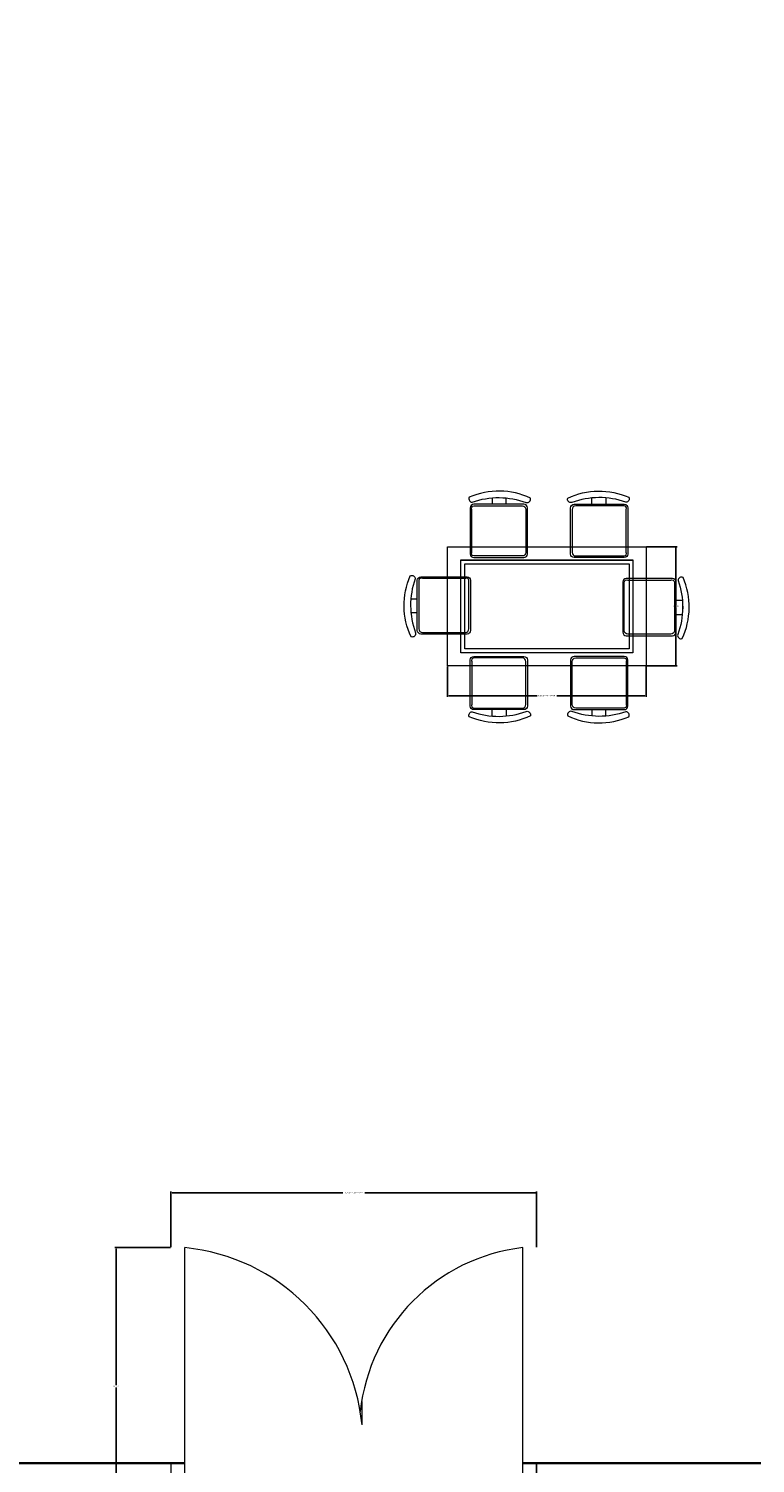
# Model space of a CAD drawing. Units: inches. Extents: x 1824 to 3509, y 619 to 2294.
# Tile 5 of 12: x 2202 to 2308, y 1115 to 1325. Entities that reach past the tile are written whole.
import ezdxf

# ---------------------------------------------------------------- set-up
doc = ezdxf.new("R2010")
doc.units = ezdxf.units.IN
for name, color, linetype, lineweight in [('A-ANNO-DIMS', 2, 'Continuous', 18), ('A-DOOR', 3, 'Continuous', 18), ('A-FURN', 8, 'Continuous', 13), ('A-WALL', 7, 'Continuous', 35)]:
    doc.layers.add(name, color=color, linetype=linetype, lineweight=lineweight)
doc.styles.get("Standard").update_dxf_attribs({"font": 'arial.ttf'})
doc.dimstyles.get("Standard").update_dxf_attribs({"dimtxt": 0.18, "dimasz": 0.18, "dimexe": 0.18, "dimexo": 0.0625, "dimgap": 0.09, "dimtad": 0, "dimtih": 1, "dimtoh": 1, "dimdec": 4, "dimzin": 0, "dimdsep": 46, "dimtxsty": 'Standard', "dimcen": 0.09, "dimadec": 0, "dimazin": 0, "dimtfac": 1, "dimtdec": 4, "dimtofl": 0, "dimtmove": 0, "dimatfit": 3, "dimfxl": 1, "dimtolj": 1, "dimtzin": 0, "dimarcsym": 0})

# ---------------------------------------------------------------- blocks, each defined once
blk = doc.blocks.new('DOOR-LOUNGE-PAIR')
for p, q in [((2, 4.5), (2, 40.5)), ((51.41, 4.5), (51.41, 40.5)), ((27.9, 14.63), (27.9, 18.05)), ((0, 9), (0, 0)), ((53.41, 0), (53.41, 9)), ((53.41, 9), (53.41, 4.5)), ((0, 0), (0, 4.5)), ((0, 4.5), (2, 4.5)), ((53.41, 4.5), (51.41, 4.5)), ((53.41, 4.5), (53.41, 4.5))]:
    blk.add_line(p, q)
for centre, radius, start, end in [((-0.78, 11.81), 28.82, 5.6014, 84.4566), ((54.5, 13.67), 27.01, 96.5732, 173.8895)]:
    blk.add_arc(centre, radius, start, end)
blk = doc.blocks.new('DINING-TABLE-PLAN')
for points in [[(0, 17.41), (29.01, 17.41), (29.01, 0), (0, 0)], [(1.93, 15.47), (27.08, 15.47), (27.08, 1.93), (1.93, 1.93)], [(2.51, 14.89), (26.5, 14.89), (26.5, 2.51), (2.51, 2.51)]]:
    blk.add_lwpolyline(points, close=True)
blk = doc.blocks.new('*D74')
at = {"layer": 'A-ANNO-DIMS', "color": 0, "lineweight": -2, "transparency": 16777216}
for p, q in [((2222.44, 1146.66), (2222.44, 1154.79)), ((2222.62, 1154.61), (2247.56, 1154.61)), ((2275.67, 1154.61), (2250.73, 1154.61)), ((2275.85, 1146.66), (2275.85, 1154.79))]:
    blk.add_line(p, q, dxfattribs=at)
at = {"layer": 'A-ANNO-DIMS', "color": 0, "transparency": 16777216}
for points in [[(2222.62, 1154.64), (2222.62, 1154.58), (2222.44, 1154.61)], [(2275.67, 1154.64), (2275.67, 1154.58), (2275.85, 1154.61)]]:
    blk.add_solid(points, dxfattribs=at)
at = {"layer": 'Defpoints', "color": 0, "transparency": 16777216}
for p in [(2275.85, 1154.61), (2222.44, 1146.6), (2275.85, 1146.6)]:
    blk.add_point(p, dxfattribs=at)
at = {"layer": 'A-ANNO-DIMS', "color": 0, "transparency": 16777216, "insert": (2249.14, 1154.61), "char_height": 0.18, "attachment_point": 5}
blk.add_mtext('\\A1;LOUNGE DOORS 53 TYP.', dxfattribs=at)
blk = doc.blocks.new('*D75')
at = {"layer": 'A-ANNO-DIMS', "color": 0, "lineweight": -2, "transparency": 16777216}
for p, q in [((2222.38, 1146.6), (2214.25, 1146.6)), ((2214.43, 1146.42), (2214.43, 1126.53)), ((2214.43, 1106.28), (2214.43, 1126.17)), ((2222.38, 1106.1), (2214.25, 1106.1))]:
    blk.add_line(p, q, dxfattribs=at)
at = {"layer": 'A-ANNO-DIMS', "color": 0, "transparency": 16777216}
for points in [[(2214.4, 1146.42), (2214.46, 1146.42), (2214.43, 1146.6)], [(2214.4, 1106.28), (2214.46, 1106.28), (2214.43, 1106.1)]]:
    blk.add_solid(points, dxfattribs=at)
at = {"layer": 'Defpoints', "color": 0, "transparency": 16777216}
for p in [(2214.43, 1146.6), (2222.44, 1146.6), (2222.44, 1106.1)]:
    blk.add_point(p, dxfattribs=at)
at = {"layer": 'A-ANNO-DIMS', "color": 0, "transparency": 16777216, "insert": (2214.43, 1126.35), "char_height": 0.18, "attachment_point": 5}
blk.add_mtext('\\A1;41 TYP.', dxfattribs=at)
blk = doc.blocks.new('*D90')
at = {"layer": 'A-ANNO-DIMS', "color": 0, "lineweight": -2, "transparency": 16777216}
for p, q in [((2262.84, 1231.49), (2262.84, 1227.02)), ((2291.85, 1231.49), (2291.85, 1227.02)), ((2263.02, 1227.2), (2275.91, 1227.2)), ((2291.67, 1227.2), (2278.78, 1227.2))]:
    blk.add_line(p, q, dxfattribs=at)
at = {"layer": 'A-ANNO-DIMS', "color": 0, "transparency": 16777216}
for points in [[(2263.02, 1227.23), (2263.02, 1227.17), (2262.84, 1227.2)], [(2291.67, 1227.23), (2291.67, 1227.17), (2291.85, 1227.2)]]:
    blk.add_solid(points, dxfattribs=at)
at = {"layer": 'Defpoints', "color": 0, "transparency": 16777216}
for p in [(2262.84, 1231.55), (2291.85, 1231.55), (2291.85, 1227.2)]:
    blk.add_point(p, dxfattribs=at)
at = {"layer": 'A-ANNO-DIMS', "color": 0, "transparency": 16777216, "insert": (2277.35, 1227.2), "char_height": 0.18, "attachment_point": 5}
blk.add_mtext('\\A1;DINING TABLE 29 TYP.', dxfattribs=at)
blk = doc.blocks.new('*D91')
at = {"layer": 'A-ANNO-DIMS', "color": 0, "lineweight": -2, "transparency": 16777216}
for p, q in [((2291.91, 1248.96), (2296.38, 1248.96)), ((2296.2, 1248.78), (2296.2, 1240.44)), ((2296.2, 1231.73), (2296.2, 1240.08)), ((2291.91, 1231.55), (2296.38, 1231.55))]:
    blk.add_line(p, q, dxfattribs=at)
at = {"layer": 'A-ANNO-DIMS', "color": 0, "transparency": 16777216}
for points in [[(2296.17, 1248.78), (2296.23, 1248.78), (2296.2, 1248.96)], [(2296.17, 1231.73), (2296.23, 1231.73), (2296.2, 1231.55)]]:
    blk.add_solid(points, dxfattribs=at)
at = {"layer": 'Defpoints', "color": 0, "transparency": 16777216}
for p in [(2291.85, 1248.96), (2296.2, 1248.96), (2291.85, 1231.55)]:
    blk.add_point(p, dxfattribs=at)
at = {"layer": 'A-ANNO-DIMS', "color": 0, "transparency": 16777216, "insert": (2296.2, 1240.26), "char_height": 0.18, "attachment_point": 5}
blk.add_mtext('\\A1;17 TYP.', dxfattribs=at)
blk = doc.blocks.new('*D94')
at = {"layer": 'A-ANNO-DIMS', "color": 0, "lineweight": -2, "transparency": 16777216}
for p, q in [((1949.09, 1049.16), (1949.09, 1668.03)), ((1949.27, 1667.85), (2235.8, 1667.85)), ((2522.91, 1667.85), (2236.38, 1667.85)), ((2523.09, 1622.16), (2523.09, 1668.03))]:
    blk.add_line(p, q, dxfattribs=at)
at = {"layer": 'A-ANNO-DIMS', "color": 0, "transparency": 16777216}
for points in [[(1949.27, 1667.88), (1949.27, 1667.82), (1949.09, 1667.85)], [(2522.91, 1667.88), (2522.91, 1667.82), (2523.09, 1667.85)]]:
    blk.add_solid(points, dxfattribs=at)
at = {"layer": 'Defpoints', "color": 0, "transparency": 16777216}
for p in [(2523.09, 1667.85), (2523.09, 1622.1), (1949.09, 1049.1)]:
    blk.add_point(p, dxfattribs=at)
at = {"layer": 'A-ANNO-DIMS', "color": 0, "transparency": 16777216, "insert": (2236.09, 1667.85), "char_height": 0.18, "attachment_point": 5}
blk.add_mtext('\\A1;574', dxfattribs=at)

msp = doc.modelspace()

# ---------------------------------------------------------------- linework, layer by layer
at = {"layer": 'A-FURN'}
for points in [[(2266.4285, 1255.4711, -0.17580919), (2274.3302, 1255.4113, 0.57839206), (2274.9288, 1256.0695, 0.21452438), (2266.0094, 1256.1892, 0.55201397), (2266.4285, 1255.4711, -0.06507904)], [(2266.4285, 1255.4708, -0.17580919), (2274.3302, 1255.411, 0.57839206), (2274.9288, 1256.0692, 0.21452438), (2266.0094, 1256.1889, 0.55201397), (2266.4285, 1255.4708, -0.06507904)], [(2280.9824, 1255.4113, -0.57839206), (2280.3838, 1256.0695, -0.21452438), (2289.3031, 1256.1892, -0.55201397), (2288.8841, 1255.4711, 0.1758092), (2280.9824, 1255.4113)], [(2280.9824, 1255.411, -0.57839206), (2280.3838, 1256.0692, -0.21452438), (2289.3031, 1256.1889, -0.55201397), (2288.8841, 1255.4708, 0.1758092), (2280.9824, 1255.411)], [(2273.9949, 1255.154), (2266.6593, 1255.154, 0.41421356), (2266.146, 1254.6408), (2266.146, 1247.8958, 0.41421356), (2266.6593, 1247.3825), (2273.9949, 1247.3825, 0.41421356), (2274.5081, 1247.8958), (2274.5081, 1254.6408, 0.41421356), (2273.9949, 1255.154)], [(2273.9949, 1255.1537), (2266.6593, 1255.1537, 0.41421356), (2266.1461, 1254.6405), (2266.1461, 1247.8954, 0.41421356), (2266.6593, 1247.3822), (2273.9949, 1247.3822, 0.41421356), (2274.5082, 1247.8954), (2274.5082, 1254.6405, 0.41421356), (2273.9949, 1255.1537)], [(2271.4183, 1255.154), (2271.4183, 1256.0817, -0.06475861)], [(2271.4183, 1255.1537), (2271.4183, 1256.0814, -0.06475861)], [(2288.6533, 1255.154, -0.41421356), (2289.1665, 1254.6408), (2289.1665, 1247.8958, -0.41421356), (2288.6533, 1247.3825), (2281.3176, 1247.3825, -0.41421356), (2280.8044, 1247.8958), (2280.8044, 1254.6408, -0.41421356), (2281.3176, 1255.154), (2288.6533, 1255.154)], [(2288.6533, 1255.1537, -0.41421356), (2289.1665, 1254.6405), (2289.1665, 1247.8954, -0.41421356), (2288.6533, 1247.3822), (2281.3176, 1247.3822, -0.41421356), (2280.8044, 1247.8954), (2280.8044, 1254.6405, -0.41421356), (2281.3176, 1255.1537), (2288.6533, 1255.1537)], [(2283.8943, 1255.154), (2283.8943, 1256.0817, 0.06475861)], [(2283.8943, 1255.1537), (2283.8943, 1256.0814, 0.06475861)], [(2258.1618, 1236.3897, -0.57839206), (2257.5035, 1235.7911, -0.21452438), (2257.3839, 1244.7104, -0.55201397), (2258.1019, 1244.2914, 0.17580937), (2258.1618, 1236.3897)], [(2258.1618, 1236.3894, -0.57839206), (2257.5036, 1235.7908, -0.21452438), (2257.3839, 1244.7101, -0.55201397), (2258.1019, 1244.2911, 0.17580937), (2258.1618, 1236.3894)], [(2258.4191, 1244.0606, -0.41421356), (2258.9323, 1244.5738), (2265.6773, 1244.5738, -0.41421356), (2266.1905, 1244.0606), (2266.1905, 1236.7249, -0.41421356), (2265.6773, 1236.2117), (2258.9323, 1236.2117, -0.41421356), (2258.4191, 1236.7249), (2258.4191, 1244.0606)], [(2258.4191, 1244.0603, -0.41421356), (2258.9323, 1244.5735), (2265.6773, 1244.5735, -0.41421356), (2266.1905, 1244.0603), (2266.1905, 1236.7246, -0.41421356), (2265.6773, 1236.2114), (2258.9323, 1236.2114, -0.41421356), (2258.4191, 1236.7246), (2258.4191, 1244.0603)], [(2296.5115, 1244.0402, -0.17580919), (2296.4516, 1236.1385, 0.57839206), (2297.1099, 1235.5399, 0.21452438), (2297.2295, 1244.4592, 0.55201397), (2296.5115, 1244.0402, -0.06507904)], [(2296.5115, 1244.0399, -0.17580919), (2296.4517, 1236.1382, 0.57839206), (2297.1099, 1235.5396, 0.21452438), (2297.2296, 1244.4589, 0.55201397), (2296.5115, 1244.0399, -0.06507904)], [(2296.1943, 1243.8094, 0.41421356), (2295.6811, 1244.3226), (2288.9361, 1244.3226, 0.41421356), (2288.4229, 1243.8094), (2288.4229, 1236.4737, 0.41421356), (2288.9361, 1235.9605), (2295.6811, 1235.9605, 0.41421356), (2296.1943, 1236.4737), (2296.1943, 1243.8094)], [(2296.1944, 1243.8091, 0.41421356), (2295.6812, 1244.3223), (2288.9361, 1244.3223, 0.41421356), (2288.4229, 1243.8091), (2288.4229, 1236.4734, 0.41421356), (2288.9361, 1235.9602), (2295.6812, 1235.9602, 0.41421356), (2296.1944, 1236.4734), (2296.1944, 1243.8091)], [(2258.4191, 1239.3016), (2257.4913, 1239.3016, 0.06475861)], [(2258.4191, 1239.3013), (2257.4913, 1239.3013, 0.06475861)], [(2296.1943, 1239.0504), (2297.1221, 1239.0504, -0.06475861)], [(2296.1944, 1239.0501), (2297.1221, 1239.0501, -0.06475861)], [(2273.9949, 1225.1708), (2266.6593, 1225.1708, -0.41421356), (2266.146, 1225.684), (2266.146, 1232.429, -0.41421356), (2266.6593, 1232.9422), (2273.9949, 1232.9422, -0.41421356), (2274.5081, 1232.429), (2274.5081, 1225.684, -0.41421356), (2273.9949, 1225.1708)], [(2273.9949, 1225.1704), (2266.6593, 1225.1704, -0.41421356), (2266.1461, 1225.6837), (2266.1461, 1232.4287, -0.41421356), (2266.6593, 1232.9419), (2273.9949, 1232.9419, -0.41421356), (2274.5082, 1232.4287), (2274.5082, 1225.6837, -0.41421356), (2273.9949, 1225.1704)], [(2288.6533, 1225.1708, 0.41421356), (2289.1665, 1225.684), (2289.1665, 1232.429, 0.41421356), (2288.6533, 1232.9422), (2281.3176, 1232.9422, 0.41421356), (2280.8044, 1232.429), (2280.8044, 1225.684, 0.41421356), (2281.3176, 1225.1708), (2288.6533, 1225.1708)], [(2288.6533, 1225.1704, 0.41421356), (2289.1665, 1225.6837), (2289.1665, 1232.4287, 0.41421356), (2288.6533, 1232.9419), (2281.3176, 1232.9419, 0.41421356), (2280.8044, 1232.4287), (2280.8044, 1225.6837, 0.41421356), (2281.3176, 1225.1704), (2288.6533, 1225.1704)], [(2274.3302, 1224.9135, -0.57839206), (2274.9288, 1224.2552, -0.21452438), (2266.0094, 1224.1356, -0.55201397), (2266.4285, 1224.8536, 0.17580929), (2274.3302, 1224.9135)], [(2274.3302, 1224.9131, -0.57839206), (2274.9288, 1224.2549, -0.21452438), (2266.0094, 1224.1352, -0.55201397), (2266.4285, 1224.8533, 0.17580929), (2274.3302, 1224.9131)], [(2271.4183, 1225.1708), (2271.4183, 1224.243, 0.06475861)], [(2271.4183, 1225.1704), (2271.4183, 1224.2427, 0.06475861)], [(2288.8841, 1224.8536, -0.17580928), (2280.9824, 1224.9135, 0.57839206), (2280.3838, 1224.2552, 0.21452438), (2289.3031, 1224.1356, 0.55201397), (2288.8841, 1224.8536, -0.06507904)], [(2288.8841, 1224.8533, -0.17580928), (2280.9824, 1224.9131, 0.57839206), (2280.3838, 1224.2549, 0.21452438), (2289.3031, 1224.1352, 0.55201397), (2288.8841, 1224.8533, -0.06507904)], [(2283.8943, 1225.1708), (2283.8943, 1224.243, -0.06475861)], [(2283.8943, 1225.1704), (2283.8943, 1224.2427, -0.06475861)]]:
    msp.add_lwpolyline(points, format="xyb", dxfattribs=at)
for points in [[(2269.3649, 1256.0986), (2269.3649, 1255.154)], [(2269.3649, 1256.0983), (2269.3649, 1255.1537)], [(2285.9476, 1256.0986), (2285.9476, 1255.154)], [(2285.9477, 1256.0983), (2285.9477, 1255.1537)], [(2257.4745, 1241.355), (2258.4191, 1241.355)], [(2257.4745, 1241.3547), (2258.4191, 1241.3547)], [(2297.1389, 1241.1037), (2296.1943, 1241.1037)], [(2297.139, 1241.1034), (2296.1944, 1241.1034)], [(2269.3649, 1224.2262), (2269.3649, 1225.1708)], [(2269.3649, 1224.2259), (2269.3649, 1225.1704)], [(2285.9476, 1224.2262), (2285.9476, 1225.1708)], [(2285.9477, 1224.2259), (2285.9477, 1225.1704)]]:
    msp.add_lwpolyline(points, dxfattribs=at)
for points in [[(2266.6624, 1254.9228), (2273.7637, 1254.9228, -0.41421356), (2274.2769, 1254.4096), (2274.2769, 1248.127, -0.41421356), (2273.7637, 1247.6137), (2266.6624, 1247.6137, -0.51206948), (2266.3773, 1248.127), (2266.3773, 1254.4096, -0.51206948)], [(2266.6624, 1254.9225), (2273.7637, 1254.9225, -0.41421356), (2274.277, 1254.4093), (2274.277, 1248.1267, -0.41421356), (2273.7637, 1247.6134), (2266.6624, 1247.6134, -0.51206948), (2266.3773, 1248.1267), (2266.3773, 1254.4093, -0.51206948)], [(2288.6502, 1254.9228), (2281.5488, 1254.9228, 0.41421356), (2281.0356, 1254.4096), (2281.0356, 1248.127, 0.41421356), (2281.5488, 1247.6137), (2288.6502, 1247.6137, 0.51206948), (2288.9353, 1248.127), (2288.9353, 1254.4096, 0.51206948)], [(2288.6502, 1254.9225), (2281.5488, 1254.9225, 0.41421356), (2281.0356, 1254.4093), (2281.0356, 1248.1267, 0.41421356), (2281.5488, 1247.6134), (2288.6502, 1247.6134, 0.51206948), (2288.9353, 1248.1267), (2288.9353, 1254.4093, 0.51206948)], [(2258.6503, 1244.0575), (2258.6503, 1236.9561, 0.41421356), (2259.1635, 1236.4429), (2265.4461, 1236.4429, 0.41421356), (2265.9593, 1236.9561), (2265.9593, 1244.0575, 0.51206948), (2265.4461, 1244.3426), (2259.1635, 1244.3426, 0.51206948)], [(2258.6503, 1244.0572), (2258.6503, 1236.9558, 0.41421356), (2259.1635, 1236.4426), (2265.4461, 1236.4426, 0.41421356), (2265.9593, 1236.9558), (2265.9593, 1244.0572, 0.51206948), (2265.4461, 1244.3423), (2259.1635, 1244.3423, 0.51206948)], [(2295.9631, 1243.8063), (2295.9631, 1236.7049, -0.41421356), (2295.4499, 1236.1917), (2289.1673, 1236.1917, -0.41421356), (2288.6541, 1236.7049), (2288.6541, 1243.8063, -0.51206948), (2289.1673, 1244.0914), (2295.4499, 1244.0914, -0.51206948)], [(2295.9632, 1243.806), (2295.9632, 1236.7046, -0.41421356), (2295.4499, 1236.1914), (2289.1673, 1236.1914, -0.41421356), (2288.6541, 1236.7046), (2288.6541, 1243.806, -0.51206948), (2289.1673, 1244.0911), (2295.4499, 1244.0911, -0.51206948)], [(2266.6624, 1225.402), (2273.7637, 1225.402, 0.41421356), (2274.2769, 1225.9152), (2274.2769, 1232.1978, 0.41421356), (2273.7637, 1232.711), (2266.6624, 1232.711, 0.51206948), (2266.3773, 1232.1978), (2266.3773, 1225.9152, 0.51206948)], [(2266.6624, 1225.4017), (2273.7637, 1225.4017, 0.41421356), (2274.277, 1225.9149), (2274.277, 1232.1975, 0.41421356), (2273.7637, 1232.7107), (2266.6624, 1232.7107, 0.51206948), (2266.3773, 1232.1975), (2266.3773, 1225.9149, 0.51206948)], [(2288.6502, 1225.402), (2281.5488, 1225.402, -0.41421356), (2281.0356, 1225.9152), (2281.0356, 1232.1978, -0.41421356), (2281.5488, 1232.711), (2288.6502, 1232.711, -0.51206948), (2288.9353, 1232.1978), (2288.9353, 1225.9152, -0.51206948)], [(2288.6502, 1225.4017), (2281.5488, 1225.4017, -0.41421356), (2281.0356, 1225.9149), (2281.0356, 1232.1975, -0.41421356), (2281.5488, 1232.7107), (2288.6502, 1232.7107, -0.51206948), (2288.9353, 1232.1975), (2288.9353, 1225.9149, -0.51206948)]]:
    msp.add_lwpolyline(points, format="xyb", close=True, dxfattribs=at)
at = {"layer": 'A-WALL'}
for p, q in [((2224.4401, 1115.1012), (2192.0899, 1115.1012)), ((2308.5899, 1115.1012), (2273.8478, 1115.1012))]:
    msp.add_line(p, q, dxfattribs=at)

# ---------------------------------------------------------------- block references
at = {"layer": 'A-DOOR'}
msp.add_blockref('DOOR-LOUNGE-PAIR', (2222.44, 1106.101), dxfattribs=at)
at = {"layer": 'A-FURN'}
for p in [(2262.84, 1231.552), (2262.84, 1231.5517)]:
    msp.add_blockref('DINING-TABLE-PLAN', p, dxfattribs=at)

# ---------------------------------------------------------------- dimensions: what is measured, and where the dimension line sits
at = {"layer": 'A-ANNO-DIMS'}
dim = msp.add_linear_dim(base=(2523.0899, 1667.8512), p1=(1949.0899, 1049.1012), p2=(2523.0899, 1622.1012), dimstyle='Standard', override={"dimdec": 0, "dimlfac": 1, "dimrnd": 0, "dimzin": 0, "dimdsep": 46, "dimlunit": 2}, dxfattribs=at)
dim.commit()
dim.dimension.update_dxf_attribs({"geometry": '*D94', "text_midpoint": (2236.0899, 1667.8512)})
for base, p1, p2, picture, middle in [((2296.2025, 1248.9588), (2291.8509, 1231.5524), (2291.8509, 1248.9588), '*D91', (2296.2025, 1240.2556)), ((2214.4289424785, 1146.6011662656), (2222.4400938008, 1106.1011662656), (2222.4400938008, 1146.6011662656), '*D75', (2214.4289424785, 1126.3511662656))]:
    dim = msp.add_linear_dim(base=base, p1=p1, p2=p2, angle=90, text='<> TYP.', dimstyle='Standard', override={"dimdec": 0, "dimlfac": 1, "dimrnd": 0, "dimzin": 0, "dimdsep": 46, "dimlunit": 2}, dxfattribs=at)
    dim.commit()
    dim.dimension.update_dxf_attribs({"geometry": picture, "text_midpoint": middle})
for base, p1, p2, text, picture, middle in [((2291.8509, 1227.2008), (2262.8401, 1231.5524), (2291.8509, 1231.5524), 'DINING TABLE <> TYP.', '*D90', (2277.3455, 1227.2008)), ((2275.8478, 1154.6123), (2222.4401, 1146.6012), (2275.8478, 1146.6012), 'LOUNGE DOORS <> TYP.', '*D74', (2249.1439, 1154.6123))]:
    dim = msp.add_linear_dim(base=base, p1=p1, p2=p2, text=text, dimstyle='Standard', override={"dimdec": 0, "dimlfac": 1, "dimrnd": 0, "dimzin": 0, "dimdsep": 46, "dimlunit": 2}, dxfattribs=at)
    dim.commit()
    dim.dimension.update_dxf_attribs({"geometry": picture, "text_midpoint": middle})

doc.saveas('drawing.dxf')
